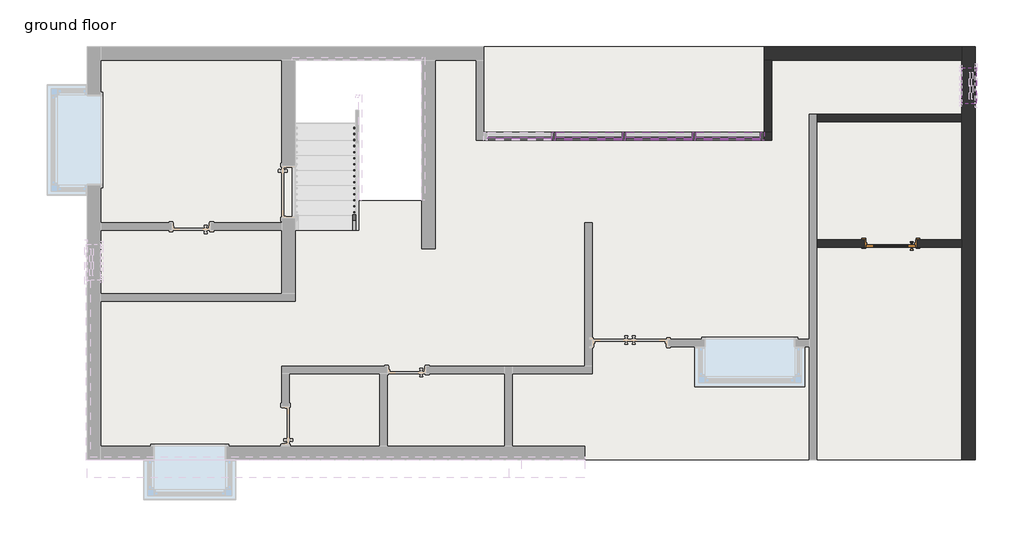
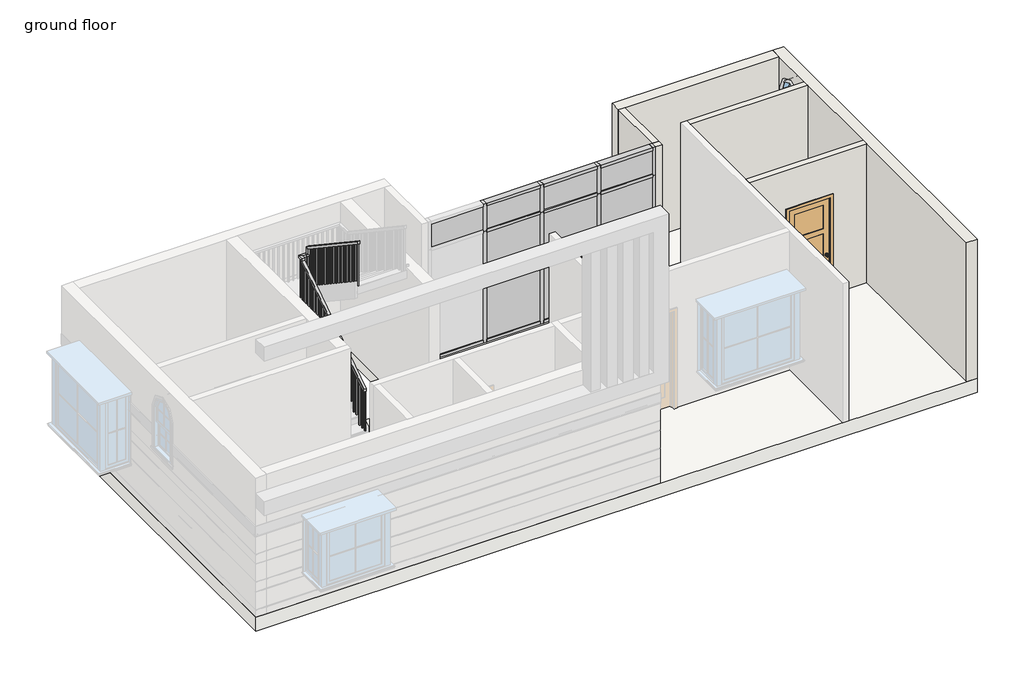
# One storey, part 4 of 5: 18 members, 7 plates, 6 walls, 1 door, 1 railing, 1 slab, 1 window.
"""IFC4 building model written with IfcOpenShell, lengths in millimetres."""

from ifc_helpers import new_model, si_unit, frame, origin, origin_with_axes, place, context, project, spatial, polyline, circle_curve, outline, extrude, faceted_brep, transform, mapped, element, save
from ifc_brep_helpers import plane_surface, revolved_surface, advanced_brep
from components import door_14766595, member_f0fea5a5, member_6e77e263, member_47bfaf8a, member_ee409385, member_5474ae84, member_211d5d53, member_0cc0e230, member_c95c5e6c, system_panel_glazed_91cb7ab6, system_panel_glazed_dcfdf68f, system_panel_glazed_3501c433, system_panel_glazed_b788c8e7, window_777a1d98

model = new_model("IFC4")

# Units and contexts
model_context = context("Model", 3, world=origin())
ifc_project = project(units=[si_unit("LENGTHUNIT", "METRE", prefix="MILLI")], contexts=[model_context])

# Site, building, storey
site = spatial("IfcSite", under=ifc_project)
building = spatial("IfcBuilding", under=site)
storey = spatial("IfcBuildingStorey", under=building, Name="ground floor", Elevation=304.8)

# Door
placement = place(None, origin())
door_shape = door_14766595(model_context)
element("IfcDoor", 1, ObjectType="Door-Interior-Single-3_Panel_Vert-Wood : 33\" x 84\"", at=placement, inside=storey, context=model_context, shape_type="MappedRepresentation", body=[
    mapped(door_shape, transform((359.1327699, -3623.5052427, 304.8), x_axis=(-1.0, 0.0, 0.0), y_axis=(0.0, -1.0, 0.0), z_axis=(0.0, 0.0, 1.0))),
])

# Members
member_shape = member_f0fea5a5(model_context)
element("IfcMember", 2, ObjectType="Rectangular Mullion : 2.5\" x 5\" rectangular", at=placement, inside=storey, context=model_context, shape_type="MappedRepresentation", body=[
    mapped(member_shape, transform((-2955.5672303, -1816.9302427, 304.8), x_axis=(-1.0, 0.0, 0.0), y_axis=(0.0, 1.0, 0.0), z_axis=(0.0, 0.0, -1.0))),
])
element("IfcMember", 3, ObjectType="Rectangular Mullion : 2.5\" x 5\" rectangular", at=placement, inside=storey, context=model_context, shape_type="MappedRepresentation", body=[
    mapped(member_shape, transform((-4136.6672301, -1816.9302427, 304.8), x_axis=(-1.0, 0.0, 0.0), y_axis=(0.0, 1.0, 0.0), z_axis=(0.0, 0.0, -1.0))),
])
element("IfcMember", 4, ObjectType="Rectangular Mullion : 2.5\" x 5\" rectangular", at=placement, inside=storey, context=model_context, shape_type="MappedRepresentation", body=[
    mapped(member_shape, transform((-5317.76723, -1816.9302427, 304.8), x_axis=(-1.0, 0.0, 0.0), y_axis=(0.0, 1.0, 0.0), z_axis=(0.0, 0.0, -1.0))),
])
member_2_shape = member_6e77e263(model_context)
element("IfcMember", 5, ObjectType="Rectangular Mullion : 2.5\" x 5\" rectangular", at=placement, inside=storey, context=model_context, shape_type="MappedRepresentation", body=[
    mapped(member_2_shape, transform((-2955.5672303, -1816.9302427, 2743.2), x_axis=(-1.0, 0.0, 0.0), y_axis=(0.0, 1.0, 0.0), z_axis=(0.0, 0.0, -1.0))),
])
element("IfcMember", 6, ObjectType="Rectangular Mullion : 2.5\" x 5\" rectangular", at=placement, inside=storey, context=model_context, shape_type="MappedRepresentation", body=[
    mapped(member_2_shape, transform((-4136.6672301, -1816.9302427, 2743.2), x_axis=(-1.0, 0.0, 0.0), y_axis=(0.0, 1.0, 0.0), z_axis=(0.0, 0.0, -1.0))),
])
element("IfcMember", 7, ObjectType="Rectangular Mullion : 2.5\" x 5\" rectangular", at=placement, inside=storey, context=model_context, shape_type="MappedRepresentation", body=[
    mapped(member_2_shape, transform((-5317.76723, -1816.9302427, 2743.2), x_axis=(-1.0, 0.0, 0.0), y_axis=(0.0, 1.0, 0.0), z_axis=(0.0, 0.0, -1.0))),
])
member_3_shape = member_47bfaf8a(model_context)
element("IfcMember", 8, ObjectType="Rectangular Mullion : 2.5\" x 5\" rectangular", at=placement, inside=storey, context=model_context, shape_type="MappedRepresentation", body=[
    mapped(member_3_shape, transform((-1774.4672301, -1816.9302427, 3352.8), x_axis=(1.0, 0.0, 0.0), y_axis=(0.0, 1.0, 0.0), z_axis=(0.0, 0.0, 1.0))),
])
member_4_shape = member_ee409385(model_context)
element("IfcMember", 9, ObjectType="Rectangular Mullion : 2.5\" x 5\" rectangular", at=placement, inside=storey, context=model_context, shape_type="MappedRepresentation", body=[
    mapped(member_4_shape, transform((-1774.4672301, -1816.9302427, 2743.2), x_axis=(1.0, 0.0, 0.0), y_axis=(0.0, 1.0, 0.0), z_axis=(0.0, 0.0, 1.0))),
])
member_5_shape = member_5474ae84(model_context)
element("IfcMember", 10, ObjectType="Rectangular Mullion : 2.5\" x 5\" rectangular", at=placement, inside=storey, context=model_context, shape_type="MappedRepresentation", body=[
    mapped(member_5_shape, transform((-2923.8172303, -1816.9302427, 3352.8), x_axis=(0.0, 0.0, 1.0), y_axis=(0.0, 1.0, 0.0), z_axis=(-1.0, 0.0, 0.0))),
])
member_6_shape = member_211d5d53(model_context)
element("IfcMember", 11, ObjectType="Rectangular Mullion : 2.5\" x 5\" rectangular", at=placement, inside=storey, context=model_context, shape_type="MappedRepresentation", body=[
    mapped(member_6_shape, transform((-4104.9172301, -1816.9302427, 3352.8), x_axis=(0.0, 0.0, 1.0), y_axis=(0.0, 1.0, 0.0), z_axis=(-1.0, 0.0, 0.0))),
])
element("IfcMember", 12, ObjectType="Rectangular Mullion : 2.5\" x 5\" rectangular", at=placement, inside=storey, context=model_context, shape_type="MappedRepresentation", body=[
    mapped(member_6_shape, transform((-5286.01723, -1816.9302427, 3352.8), x_axis=(0.0, 0.0, 1.0), y_axis=(0.0, 1.0, 0.0), z_axis=(-1.0, 0.0, 0.0))),
])
element("IfcMember", 13, ObjectType="Rectangular Mullion : 2.5\" x 5\" rectangular", at=placement, inside=storey, context=model_context, shape_type="MappedRepresentation", body=[
    mapped(member_5_shape, transform((-1837.9672301, -1816.9302427, 304.8), x_axis=(0.0, 0.0, -1.0), y_axis=(0.0, 1.0, 0.0), z_axis=(1.0, 0.0, 0.0))),
])
element("IfcMember", 14, ObjectType="Rectangular Mullion : 2.5\" x 5\" rectangular", at=placement, inside=storey, context=model_context, shape_type="MappedRepresentation", body=[
    mapped(member_5_shape, transform((-5349.51723, -1816.9302427, 304.8), x_axis=(0.0, 0.0, -1.0), y_axis=(0.0, 1.0, 0.0), z_axis=(1.0, 0.0, 0.0))),
])
element("IfcMember", 15, ObjectType="Rectangular Mullion : 2.5\" x 5\" rectangular", at=placement, inside=storey, context=model_context, shape_type="MappedRepresentation", body=[
    mapped(member_6_shape, transform((-2987.3172303, -1816.9302427, 304.8), x_axis=(0.0, 0.0, -1.0), y_axis=(0.0, 1.0, 0.0), z_axis=(1.0, 0.0, 0.0))),
])
element("IfcMember", 16, ObjectType="Rectangular Mullion : 2.5\" x 5\" rectangular", at=placement, inside=storey, context=model_context, shape_type="MappedRepresentation", body=[
    mapped(member_6_shape, transform((-4168.4172301, -1816.9302427, 304.8), x_axis=(0.0, 0.0, -1.0), y_axis=(0.0, 1.0, 0.0), z_axis=(1.0, 0.0, 0.0))),
])
member_7_shape = member_0cc0e230(model_context)
element("IfcMember", 17, ObjectType="Rectangular Mullion : 2.5\" x 5\" rectangular", at=placement, inside=storey, context=model_context, shape_type="MappedRepresentation", body=[
    mapped(member_7_shape, transform((-2923.8172303, -1816.9302427, 2743.2), x_axis=(0.0, 0.0, 1.0), y_axis=(0.0, 1.0, 0.0), z_axis=(-1.0, 0.0, 0.0))),
])
member_8_shape = member_c95c5e6c(model_context)
element("IfcMember", 18, ObjectType="Rectangular Mullion : 2.5\" x 5\" rectangular", at=placement, inside=storey, context=model_context, shape_type="MappedRepresentation", body=[
    mapped(member_8_shape, transform((-4104.9172301, -1816.9302427, 2743.2), x_axis=(0.0, 0.0, 1.0), y_axis=(0.0, 1.0, 0.0), z_axis=(-1.0, 0.0, 0.0))),
])
element("IfcMember", 19, ObjectType="Rectangular Mullion : 2.5\" x 5\" rectangular", at=placement, inside=storey, context=model_context, shape_type="MappedRepresentation", body=[
    mapped(member_8_shape, transform((-5286.01723, -1816.9302427, 2743.2), x_axis=(0.0, 0.0, 1.0), y_axis=(0.0, 1.0, 0.0), z_axis=(-1.0, 0.0, 0.0))),
])

# Plates
system_panel_glazed_shape = system_panel_glazed_91cb7ab6(model_context)
element("IfcPlate", 20, ObjectType="System Panel : Glazed", at=placement, inside=storey, context=model_context, shape_type="MappedRepresentation", body=[
    mapped(system_panel_glazed_shape, transform((-2380.8922302, -1816.9302427, 368.3), x_axis=(-1.0, 0.0, 0.0), y_axis=(0.0, -1.0, 0.0), z_axis=(0.0, 0.0, 1.0))),
])
system_panel_glazed_2_shape = system_panel_glazed_dcfdf68f(model_context)
element("IfcPlate", 21, ObjectType="System Panel : Glazed", at=placement, inside=storey, context=model_context, shape_type="MappedRepresentation", body=[
    mapped(system_panel_glazed_2_shape, transform((-3546.1172302, -1816.9302427, 368.3), x_axis=(-1.0, 0.0, 0.0), y_axis=(0.0, -1.0, 0.0), z_axis=(0.0, 0.0, 1.0))),
])
element("IfcPlate", 22, ObjectType="System Panel : Glazed", at=placement, inside=storey, context=model_context, shape_type="MappedRepresentation", body=[
    mapped(system_panel_glazed_2_shape, transform((-4727.21723, -1816.9302427, 368.3), x_axis=(-1.0, 0.0, 0.0), y_axis=(0.0, -1.0, 0.0), z_axis=(0.0, 0.0, 1.0))),
])
system_panel_glazed_3_shape = system_panel_glazed_3501c433(model_context)
element("IfcPlate", 23, ObjectType="System Panel : Glazed", at=placement, inside=storey, context=model_context, shape_type="MappedRepresentation", body=[
    mapped(system_panel_glazed_3_shape, transform((-2380.8922302, -1816.9302427, 2774.95), x_axis=(-1.0, 0.0, 0.0), y_axis=(0.0, -1.0, 0.0), z_axis=(0.0, 0.0, 1.0))),
])
element("IfcPlate", 24, ObjectType="System Panel : Glazed", at=placement, inside=storey, context=model_context, shape_type="MappedRepresentation", body=[
    mapped(system_panel_glazed_3_shape, transform((-5892.44223, -1816.9302427, 2774.95), x_axis=(-1.0, 0.0, 0.0), y_axis=(0.0, -1.0, 0.0), z_axis=(0.0, 0.0, 1.0))),
])
system_panel_glazed_4_shape = system_panel_glazed_b788c8e7(model_context)
element("IfcPlate", 25, ObjectType="System Panel : Glazed", at=placement, inside=storey, context=model_context, shape_type="MappedRepresentation", body=[
    mapped(system_panel_glazed_4_shape, transform((-3546.1172302, -1816.9302427, 2774.95), x_axis=(-1.0, 0.0, 0.0), y_axis=(0.0, -1.0, 0.0), z_axis=(0.0, 0.0, 1.0))),
])
element("IfcPlate", 26, ObjectType="System Panel : Glazed", at=placement, inside=storey, context=model_context, shape_type="MappedRepresentation", body=[
    mapped(system_panel_glazed_4_shape, transform((-4727.21723, -1816.9302427, 2774.95), x_axis=(-1.0, 0.0, 0.0), y_axis=(0.0, -1.0, 0.0), z_axis=(0.0, 0.0, 1.0))),
])

# Railing
element("IfcRailing", 27, ObjectType="Handrail - Rectangular", at=placement, inside=storey, context=model_context, shape_type="SolidModel", body=[
    faceted_brep([(-8708.6672301, -3404.4302427, 1388.5333333), (-8708.6672301, -3404.4302427, 1327.4793317), (-8657.8672301, -3404.4302427, 1327.4793317), (-8657.8672301, -3404.4302427, 1388.5333333), (-8708.6672301, -1194.6302427, 2861.7333333), (-8708.6672301, -1143.8302427, 2834.5459984), (-8657.8672301, -1143.8302427, 2834.5459984), (-8657.8672301, -1194.6302427, 2861.7333333), (-8708.6672301, -1194.6302427, 2912.5333333), (-8708.6672301, -1143.8302427, 2861.7333333), (-8657.8672301, -1143.8302427, 2861.7333333), (-8657.8672301, -1194.6302427, 2912.5333333), (-8708.6672301, -1067.6302427, 2912.5333333), (-8708.6672301, -1067.6302427, 2861.7333333), (-8657.8672301, -1118.4302427, 2861.7333333), (-8657.8672301, -1118.4302427, 2912.5333333), (-8581.6672301, -1067.6302427, 2912.5333333), (-8581.6672301, -1067.6302427, 2861.7333333), (-8581.6672301, -1118.4302427, 2861.7333333), (-8581.6672301, -1118.4302427, 2912.5333333), (-8556.2672301, -1067.6302427, 2912.5333333), (-8556.2672301, -1118.4302427, 2912.5333333), (-8505.4672301, -1118.4302427, 2861.7333333), (-8505.4672301, -1067.6302427, 2861.7333333)], [[[0, 1, 2, 3]], [[1, 0, 4, 5]], [[2, 1, 5, 6]], [[3, 2, 6, 7]], [[0, 3, 7, 4]], [[5, 4, 8, 9]], [[6, 5, 9, 10]], [[7, 6, 10, 11]], [[4, 7, 11, 8]], [[9, 8, 12, 13]], [[10, 9, 13, 14]], [[11, 10, 14, 15]], [[8, 11, 15, 12]], [[13, 12, 16, 17]], [[14, 13, 17, 18]], [[15, 14, 18, 19]], [[12, 15, 19, 16]], [[20, 21, 22, 23]], [[17, 16, 20, 23]], [[18, 17, 23, 22]], [[19, 18, 22, 21]], [[16, 19, 21, 20]]]),
    faceted_brep([(-8556.2672301, -1067.6302427, 2912.5333333), (-8505.4672301, -1067.6302427, 2861.7333333), (-8505.4672301, -1118.4302427, 2861.7333333), (-8556.2672301, -1118.4302427, 2912.5333333), (-8556.2672301, -1067.6302427, 3048.0), (-8556.2672301, -1118.4302427, 3020.8126651), (-8505.4672301, -1118.4302427, 3020.8126651), (-8505.4672301, -1067.6302427, 3048.0)], [[[0, 1, 2, 3]], [[4, 5, 6, 7]], [[1, 0, 4, 7]], [[2, 1, 7, 6]], [[3, 2, 6, 5]], [[0, 3, 5, 4]]]),
    faceted_brep([(-8505.4672301, -1067.6302427, 3048.0), (-8505.4672301, -1118.4302427, 3020.8126651), (-8556.2672301, -1118.4302427, 3020.8126651), (-8556.2672301, -1067.6302427, 3048.0), (-8505.4672301, -2896.4302427, 4267.2), (-8556.2672301, -2896.4302427, 4267.2), (-8556.2672301, -2896.4302427, 4206.1459984), (-8505.4672301, -2896.4302427, 4206.1459984)], [[[0, 1, 2, 3]], [[4, 5, 6, 7]], [[1, 0, 4, 7]], [[2, 1, 7, 6]], [[3, 2, 6, 5]], [[0, 3, 5, 4]]]),
    extrude(outline(polyline([(-2829.7552427, 4161.6959984), (-2810.7052427, 4148.9959984), (-2810.7052427, 3183.4666667), (-2829.7552427, 3183.4666667), (-2829.7552427, 4161.6959984)])), frame((-8540.3922301, 0.0, 0.0), z_axis=(1.0, 0.0, 0.0), x_axis=(0.0, 1.0, 0.0)), (0.0, 0.0, 1.0), 19.05),
    extrude(outline(polyline([(-2728.1552427, 4093.9626651), (-2709.1052427, 4081.2626651), (-2709.1052427, 3183.4666667), (-2728.1552427, 3183.4666667), (-2728.1552427, 4093.9626651)])), frame((-8540.3922301, 0.0, 0.0), z_axis=(1.0, 0.0, 0.0), x_axis=(0.0, 1.0, 0.0)), (0.0, 0.0, 1.0), 19.05),
    extrude(outline(polyline([(-2626.5552427, 4026.2293317), (-2607.5052427, 4013.5293317), (-2607.5052427, 3014.1333333), (-2626.5552427, 3014.1333333), (-2626.5552427, 4026.2293317)])), frame((-8540.3922301, 0.0, 0.0), z_axis=(1.0, 0.0, 0.0), x_axis=(0.0, 1.0, 0.0)), (0.0, 0.0, 1.0), 19.05),
    extrude(outline(polyline([(-2524.9552427, 3958.4959984), (-2505.9052427, 3945.7959984), (-2505.9052427, 3014.1333333), (-2524.9552427, 3014.1333333), (-2524.9552427, 3958.4959984)])), frame((-8540.3922301, 0.0, 0.0), z_axis=(1.0, 0.0, 0.0), x_axis=(0.0, 1.0, 0.0)), (0.0, 0.0, 1.0), 19.05),
    extrude(outline(polyline([(-2423.3552427, 3890.7626651), (-2404.3052427, 3878.0626651), (-2404.3052427, 3014.1333333), (-2423.3552427, 3014.1333333), (-2423.3552427, 3890.7626651)])), frame((-8540.3922301, 0.0, 0.0), z_axis=(1.0, 0.0, 0.0), x_axis=(0.0, 1.0, 0.0)), (0.0, 0.0, 1.0), 19.05),
    extrude(outline(polyline([(-2321.7552427, 3823.0293317), (-2302.7052427, 3810.3293317), (-2302.7052427, 2844.8), (-2321.7552427, 2844.8), (-2321.7552427, 3823.0293317)])), frame((-8540.3922301, 0.0, 0.0), z_axis=(1.0, 0.0, 0.0), x_axis=(0.0, 1.0, 0.0)), (0.0, 0.0, 1.0), 19.05),
    extrude(outline(polyline([(-2220.1552427, 3755.2959984), (-2201.1052427, 3742.5959984), (-2201.1052427, 2844.8), (-2220.1552427, 2844.8), (-2220.1552427, 3755.2959984)])), frame((-8540.3922301, 0.0, 0.0), z_axis=(1.0, 0.0, 0.0), x_axis=(0.0, 1.0, 0.0)), (0.0, 0.0, 1.0), 19.05),
    extrude(outline(polyline([(-2118.5552427, 3687.5626651), (-2099.5052427, 3674.8626651), (-2099.5052427, 2675.4666667), (-2118.5552427, 2675.4666667), (-2118.5552427, 3687.5626651)])), frame((-8540.3922301, 0.0, 0.0), z_axis=(1.0, 0.0, 0.0), x_axis=(0.0, 1.0, 0.0)), (0.0, 0.0, 1.0), 19.05),
    extrude(outline(polyline([(-2016.9552427, 3619.8293317), (-1997.9052427, 3607.1293317), (-1997.9052427, 2675.4666667), (-2016.9552427, 2675.4666667), (-2016.9552427, 3619.8293317)])), frame((-8540.3922301, 0.0, 0.0), z_axis=(1.0, 0.0, 0.0), x_axis=(0.0, 1.0, 0.0)), (0.0, 0.0, 1.0), 19.05),
    extrude(outline(polyline([(-1915.3552427, 3552.0959984), (-1896.3052427, 3539.3959984), (-1896.3052427, 2675.4666667), (-1915.3552427, 2675.4666667), (-1915.3552427, 3552.0959984)])), frame((-8540.3922301, 0.0, 0.0), z_axis=(1.0, 0.0, 0.0), x_axis=(0.0, 1.0, 0.0)), (0.0, 0.0, 1.0), 19.05),
    extrude(outline(polyline([(-1813.7552427, 3484.3626651), (-1794.7052427, 3471.6626651), (-1794.7052427, 2506.1333333), (-1813.7552427, 2506.1333333), (-1813.7552427, 3484.3626651)])), frame((-8540.3922301, 0.0, 0.0), z_axis=(1.0, 0.0, 0.0), x_axis=(0.0, 1.0, 0.0)), (0.0, 0.0, 1.0), 19.05),
    extrude(outline(polyline([(-1712.1552427, 3416.6293317), (-1693.1052427, 3403.9293317), (-1693.1052427, 2506.1333333), (-1712.1552427, 2506.1333333), (-1712.1552427, 3416.6293317)])), frame((-8540.3922301, 0.0, 0.0), z_axis=(1.0, 0.0, 0.0), x_axis=(0.0, 1.0, 0.0)), (0.0, 0.0, 1.0), 19.05),
    extrude(outline(polyline([(-1610.5552427, 3348.8959984), (-1591.5052427, 3336.1959984), (-1591.5052427, 2336.8), (-1610.5552427, 2336.8), (-1610.5552427, 3348.8959984)])), frame((-8540.3922301, 0.0, 0.0), z_axis=(1.0, 0.0, 0.0), x_axis=(0.0, 1.0, 0.0)), (0.0, 0.0, 1.0), 19.05),
    extrude(outline(polyline([(-1508.9552427, 3281.1626651), (-1489.9052427, 3268.4626651), (-1489.9052427, 2336.8), (-1508.9552427, 2336.8), (-1508.9552427, 3281.1626651)])), frame((-8540.3922301, 0.0, 0.0), z_axis=(1.0, 0.0, 0.0), x_axis=(0.0, 1.0, 0.0)), (0.0, 0.0, 1.0), 19.05),
    extrude(outline(polyline([(-1407.3552427, 3213.4293317), (-1388.3052427, 3200.7293317), (-1388.3052427, 2336.8), (-1407.3552427, 2336.8), (-1407.3552427, 3213.4293317)])), frame((-8540.3922301, 0.0, 0.0), z_axis=(1.0, 0.0, 0.0), x_axis=(0.0, 1.0, 0.0)), (0.0, 0.0, 1.0), 19.05),
    extrude(outline(polyline([(-1305.7552427, 3145.6959984), (-1286.7052427, 3132.9959984), (-1286.7052427, 2167.4666667), (-1305.7552427, 2167.4666667), (-1305.7552427, 3145.6959984)])), frame((-8540.3922301, 0.0, 0.0), z_axis=(1.0, 0.0, 0.0), x_axis=(0.0, 1.0, 0.0)), (0.0, 0.0, 1.0), 19.05),
    extrude(outline(polyline([(-1204.1552427, 3077.9626651), (-1185.1052427, 3065.2626651), (-1185.1052427, 2167.4666667), (-1204.1552427, 2167.4666667), (-1204.1552427, 3077.9626651)])), frame((-8540.3922301, 0.0, 0.0), z_axis=(1.0, 0.0, 0.0), x_axis=(0.0, 1.0, 0.0)), (0.0, 0.0, 1.0), 19.05),
    extrude(outline(polyline([(-8591.1922301, -1102.5552427), (-8591.1922301, -1083.5052427), (-8572.1422301, -1083.5052427), (-8572.1422301, -1102.5552427), (-8591.1922301, -1102.5552427)])), frame((0.0, 0.0, 1998.1333333), z_axis=(0.0, 0.0, 1.0), x_axis=(1.0, 0.0, 0.0)), (0.0, 0.0, 1.0), 863.6),
    extrude(outline(polyline([(-8673.7422301, -1178.7552427), (-8692.7922301, -1178.7552427), (-8692.7922301, -1159.7052427), (-8673.7422301, -1159.7052427), (-8673.7422301, -1178.7552427)])), frame((0.0, 0.0, 1828.8), z_axis=(0.0, 0.0, 1.0), x_axis=(1.0, 0.0, 0.0)), (0.0, 0.0, 1.0), 1032.9333333),
    extrude(outline(polyline([(-1280.3552427, 2743.5293317), (-1261.3052427, 2756.2293317), (-1261.3052427, 1828.8), (-1280.3552427, 1828.8), (-1280.3552427, 2743.5293317)])), frame((-8692.7922301, 0.0, 0.0), z_axis=(1.0, 0.0, 0.0), x_axis=(0.0, 1.0, 0.0)), (0.0, 0.0, 1.0), 19.05),
    extrude(outline(polyline([(-1381.9552427, 2675.7959984), (-1362.9052427, 2688.4959984), (-1362.9052427, 1828.8), (-1381.9552427, 1828.8), (-1381.9552427, 2675.7959984)])), frame((-8692.7922301, 0.0, 0.0), z_axis=(1.0, 0.0, 0.0), x_axis=(0.0, 1.0, 0.0)), (0.0, 0.0, 1.0), 19.05),
    extrude(outline(polyline([(-1483.5552427, 2608.0626651), (-1464.5052427, 2620.7626651), (-1464.5052427, 1659.4666667), (-1483.5552427, 1659.4666667), (-1483.5552427, 2608.0626651)])), frame((-8692.7922301, 0.0, 0.0), z_axis=(1.0, 0.0, 0.0), x_axis=(0.0, 1.0, 0.0)), (0.0, 0.0, 1.0), 19.05),
    extrude(outline(polyline([(-1585.1552427, 2540.3293317), (-1566.1052427, 2553.0293317), (-1566.1052427, 1659.4666667), (-1585.1552427, 1659.4666667), (-1585.1552427, 2540.3293317)])), frame((-8692.7922301, 0.0, 0.0), z_axis=(1.0, 0.0, 0.0), x_axis=(0.0, 1.0, 0.0)), (0.0, 0.0, 1.0), 19.05),
    extrude(outline(polyline([(-1686.7552427, 2472.5959984), (-1667.7052427, 2485.2959984), (-1667.7052427, 1490.1333333), (-1686.7552427, 1490.1333333), (-1686.7552427, 2472.5959984)])), frame((-8692.7922301, 0.0, 0.0), z_axis=(1.0, 0.0, 0.0), x_axis=(0.0, 1.0, 0.0)), (0.0, 0.0, 1.0), 19.05),
    extrude(outline(polyline([(-1788.3552427, 2404.8626651), (-1769.3052427, 2417.5626651), (-1769.3052427, 1490.1333333), (-1788.3552427, 1490.1333333), (-1788.3552427, 2404.8626651)])), frame((-8692.7922301, 0.0, 0.0), z_axis=(1.0, 0.0, 0.0), x_axis=(0.0, 1.0, 0.0)), (0.0, 0.0, 1.0), 19.05),
    extrude(outline(polyline([(-1889.9552427, 2337.1293317), (-1870.9052427, 2349.8293317), (-1870.9052427, 1490.1333333), (-1889.9552427, 1490.1333333), (-1889.9552427, 2337.1293317)])), frame((-8692.7922301, 0.0, 0.0), z_axis=(1.0, 0.0, 0.0), x_axis=(0.0, 1.0, 0.0)), (0.0, 0.0, 1.0), 19.05),
    extrude(outline(polyline([(-1991.5552427, 2269.3959984), (-1972.5052427, 2282.0959984), (-1972.5052427, 1320.8), (-1991.5552427, 1320.8), (-1991.5552427, 2269.3959984)])), frame((-8692.7922301, 0.0, 0.0), z_axis=(1.0, 0.0, 0.0), x_axis=(0.0, 1.0, 0.0)), (0.0, 0.0, 1.0), 19.05),
    extrude(outline(polyline([(-2093.1552427, 2201.6626651), (-2074.1052427, 2214.3626651), (-2074.1052427, 1320.8), (-2093.1552427, 1320.8), (-2093.1552427, 2201.6626651)])), frame((-8692.7922301, 0.0, 0.0), z_axis=(1.0, 0.0, 0.0), x_axis=(0.0, 1.0, 0.0)), (0.0, 0.0, 1.0), 19.05),
    extrude(outline(polyline([(-2194.7552427, 2133.9293317), (-2175.7052427, 2146.6293317), (-2175.7052427, 1151.4666667), (-2194.7552427, 1151.4666667), (-2194.7552427, 2133.9293317)])), frame((-8692.7922301, 0.0, 0.0), z_axis=(1.0, 0.0, 0.0), x_axis=(0.0, 1.0, 0.0)), (0.0, 0.0, 1.0), 19.05),
    extrude(outline(polyline([(-2296.3552427, 2066.1959984), (-2277.3052427, 2078.8959984), (-2277.3052427, 1151.4666667), (-2296.3552427, 1151.4666667), (-2296.3552427, 2066.1959984)])), frame((-8692.7922301, 0.0, 0.0), z_axis=(1.0, 0.0, 0.0), x_axis=(0.0, 1.0, 0.0)), (0.0, 0.0, 1.0), 19.05),
    extrude(outline(polyline([(-2397.9552427, 1998.4626651), (-2378.9052427, 2011.1626651), (-2378.9052427, 1151.4666667), (-2397.9552427, 1151.4666667), (-2397.9552427, 1998.4626651)])), frame((-8692.7922301, 0.0, 0.0), z_axis=(1.0, 0.0, 0.0), x_axis=(0.0, 1.0, 0.0)), (0.0, 0.0, 1.0), 19.05),
    extrude(outline(polyline([(-2499.5552427, 1930.7293317), (-2480.5052427, 1943.4293317), (-2480.5052427, 982.1333333), (-2499.5552427, 982.1333333), (-2499.5552427, 1930.7293317)])), frame((-8692.7922301, 0.0, 0.0), z_axis=(1.0, 0.0, 0.0), x_axis=(0.0, 1.0, 0.0)), (0.0, 0.0, 1.0), 19.05),
    extrude(outline(polyline([(-2601.1552427, 1862.9959984), (-2582.1052427, 1875.6959984), (-2582.1052427, 982.1333333), (-2601.1552427, 982.1333333), (-2601.1552427, 1862.9959984)])), frame((-8692.7922301, 0.0, 0.0), z_axis=(1.0, 0.0, 0.0), x_axis=(0.0, 1.0, 0.0)), (0.0, 0.0, 1.0), 19.05),
    extrude(outline(polyline([(-2702.7552427, 1795.2626651), (-2683.7052427, 1807.9626651), (-2683.7052427, 812.8), (-2702.7552427, 812.8), (-2702.7552427, 1795.2626651)])), frame((-8692.7922301, 0.0, 0.0), z_axis=(1.0, 0.0, 0.0), x_axis=(0.0, 1.0, 0.0)), (0.0, 0.0, 1.0), 19.05),
    extrude(outline(polyline([(-2804.3552427, 1727.5293317), (-2785.3052427, 1740.2293317), (-2785.3052427, 812.8), (-2804.3552427, 812.8), (-2804.3552427, 1727.5293317)])), frame((-8692.7922301, 0.0, 0.0), z_axis=(1.0, 0.0, 0.0), x_axis=(0.0, 1.0, 0.0)), (0.0, 0.0, 1.0), 19.05),
    extrude(outline(polyline([(-2905.9552427, 1659.7959984), (-2886.9052427, 1672.4959984), (-2886.9052427, 812.8), (-2905.9552427, 812.8), (-2905.9552427, 1659.7959984)])), frame((-8692.7922301, 0.0, 0.0), z_axis=(1.0, 0.0, 0.0), x_axis=(0.0, 1.0, 0.0)), (0.0, 0.0, 1.0), 19.05),
    extrude(outline(polyline([(-3007.5552427, 1592.0626651), (-2988.5052427, 1604.7626651), (-2988.5052427, 643.4666667), (-3007.5552427, 643.4666667), (-3007.5552427, 1592.0626651)])), frame((-8692.7922301, 0.0, 0.0), z_axis=(1.0, 0.0, 0.0), x_axis=(0.0, 1.0, 0.0)), (0.0, 0.0, 1.0), 19.05),
    extrude(outline(polyline([(-3109.1552427, 1524.3293317), (-3090.1052427, 1537.0293317), (-3090.1052427, 643.4666667), (-3109.1552427, 643.4666667), (-3109.1552427, 1524.3293317)])), frame((-8692.7922301, 0.0, 0.0), z_axis=(1.0, 0.0, 0.0), x_axis=(0.0, 1.0, 0.0)), (0.0, 0.0, 1.0), 19.05),
    extrude(outline(polyline([(-3210.7552427, 1456.5959984), (-3191.7052427, 1469.2959984), (-3191.7052427, 474.1333333), (-3210.7552427, 474.1333333), (-3210.7552427, 1456.5959984)])), frame((-8692.7922301, 0.0, 0.0), z_axis=(1.0, 0.0, 0.0), x_axis=(0.0, 1.0, 0.0)), (0.0, 0.0, 1.0), 19.05),
    extrude(outline(polyline([(-3312.3552427, 1388.8626651), (-3293.3052427, 1401.5626651), (-3293.3052427, 474.1333333), (-3312.3552427, 474.1333333), (-3312.3552427, 1388.8626651)])), frame((-8692.7922301, 0.0, 0.0), z_axis=(1.0, 0.0, 0.0), x_axis=(0.0, 1.0, 0.0)), (0.0, 0.0, 1.0), 19.05),
    extrude(outline(polyline([(-8540.3922301, -1102.5552427), (-8540.3922301, -1083.5052427), (-8521.3422301, -1083.5052427), (-8521.3422301, -1102.5552427), (-8540.3922301, -1102.5552427)])), frame((0.0, 0.0, 1998.1333333), z_axis=(0.0, 0.0, 1.0), x_axis=(1.0, 0.0, 0.0)), (0.0, 0.0, 1.0), 863.6),
    extrude(outline(polyline([(-8673.7422301, -1102.5552427), (-8692.7922301, -1102.5552427), (-8692.7922301, -1083.5052427), (-8673.7422301, -1083.5052427), (-8673.7422301, -1102.5552427)])), frame((0.0, 0.0, 1998.1333333), z_axis=(0.0, 0.0, 1.0), x_axis=(1.0, 0.0, 0.0)), (0.0, 0.0, 1.0), 863.6),
    extrude(outline(polyline([(-2896.4302427, 4206.1459984), (-2877.3802427, 4193.4459984), (-2877.3802427, 3183.4666667), (-2896.4302427, 3183.4666667), (-2896.4302427, 4206.1459984)])), frame((-8540.3922301, 0.0, 0.0), z_axis=(1.0, 0.0, 0.0), x_axis=(0.0, 1.0, 0.0)), (0.0, 0.0, 1.0), 19.05),
    extrude(outline(polyline([(-3404.4302427, 1327.4793317), (-3385.3802427, 1340.1793317), (-3385.3802427, 474.1333333), (-3404.4302427, 474.1333333), (-3404.4302427, 1327.4793317)])), frame((-8692.7922301, 0.0, 0.0), z_axis=(1.0, 0.0, 0.0), x_axis=(0.0, 1.0, 0.0)), (0.0, 0.0, 1.0), 19.05),
])

# Slab
element("IfcSlab", 28, ObjectType="Generic - 12\"", at=placement, inside=storey, context=model_context, shape_type="SweptSolid", body=[
    extrude(outline(polyline([(1781.5327699, -305.6302427), (1781.5327699, -7265.2302427), (-13179.0672301, -7265.2302427), (-13179.0672301, -305.6302427), (1781.5327699, -305.6302427)]), holes=[polyline([(-9724.6672301, -3379.0302427), (-8607.0672301, -3404.4302427), (-8607.0672301, -2896.4302427), (-7489.4672301, -2896.4302427), (-7489.4672301, -483.4302427), (-9724.6672301, -483.4302427), (-9724.6672301, -3379.0302427)])]), origin_with_axes(), (0.0, 0.0, 1.0), 304.8),
])

# Walls
element("IfcWall", 29, ObjectType="INNER WALL 5\"", at=placement, inside=storey, context=model_context, shape_type="SweptSolid", body=[
    extrude(outline(polyline([(1552.9327699, -1575.6302427), (-885.4672301, -1575.6302427), (-885.4672301, -1448.6302427), (1552.9327699, -1448.6302427), (1552.9327699, -1575.6302427)])), frame((0.0, 0.0, 304.8), z_axis=(0.0, 0.0, 1.0), x_axis=(1.0, 0.0, 0.0)), (0.0, 0.0, 1.0), 3048.0),
])
element("IfcWall", 30, ObjectType="INNER WALL 5\"", at=placement, inside=storey, context=model_context, shape_type="SweptSolid", body=[
    extrude(outline(polyline([(3352.8, 1552.9327699), (3352.8, -885.4672301), (304.8, -885.4672301), (304.8, -85.3672301), (2463.8, -85.3672301), (2463.8, 803.6327699), (304.8, 803.6327699), (304.8, 1552.9327699), (3352.8, 1552.9327699)])), frame((0.0, -3683.8302427, 0.0), z_axis=(0.0, 1.0, 0.0), x_axis=(0.0, 0.0, 1.0)), (0.0, 0.0, 1.0), 127.0),
])
element("IfcWall", 31, ObjectType="INNER WALL 5\"", at=placement, inside=storey, context=model_context, shape_type="SweptSolid", body=[
    extrude(outline(polyline([(-1647.4672301, -1753.4302427), (-1647.4672301, -1880.4302427), (-1774.4672301, -1880.4302427), (-1774.4672301, -1753.4302427), (-1647.4672301, -1753.4302427)])), frame((0.0, 0.0, 304.8), z_axis=(0.0, 0.0, 1.0), x_axis=(1.0, 0.0, 0.0)), (0.0, 0.0, 1.0), 3048.0),
])
element("IfcWall", 32, ObjectType="INNER WALL 5\"", at=placement, inside=storey, context=model_context, shape_type="SweptSolid", body=[
    extrude(outline(polyline([(-1647.4672301, -534.2302427), (-1647.4672301, -1753.4302427), (-1774.4672301, -1753.4302427), (-1774.4672301, -534.2302427), (-1647.4672301, -534.2302427)])), frame((0.0, 0.0, 304.8), z_axis=(0.0, 0.0, 1.0), x_axis=(1.0, 0.0, 0.0)), (0.0, 0.0, 1.0), 3048.0),
])
element("IfcWall", 33, ObjectType="OUTER WALL 9\"", at=placement, inside=storey, context=model_context, shape_type="AdvancedBrep", body=[
    advanced_brep(
    [(1781.5327699, -7265.2302427, 304.8), (1781.5327699, -305.6302427, 304.8), (1781.5327699, -305.6302427, 3352.8), (1781.5327699, -7265.2302427, 3352.8), (1781.5327699, -1270.8302427, 2743.2), (1781.5327699, -661.2302427, 2743.2), (1781.5327699, -661.2302427, 1828.8), (1781.5327699, -1270.8302427, 1828.8), (1552.9327699, -7265.2302427, 304.8), (1552.9327699, -7265.2302427, 3352.8), (1552.9327699, -3683.8302427, 3352.8), (1552.9327699, -3556.8302427, 3352.8), (1552.9327699, -1575.6302427, 3352.8), (1552.9327699, -1448.6302427, 3352.8), (1552.9327699, -534.2302427, 3352.8), (1552.9327699, -305.6302427, 3352.8), (1552.9327699, -305.6302427, 304.8), (1552.9327699, -534.2302427, 304.8), (1552.9327699, -1448.6302427, 304.8), (1552.9327699, -1575.6302427, 304.8), (1552.9327699, -3556.8302427, 304.8), (1552.9327699, -3683.8302427, 304.8), (1552.9327699, -1270.8302427, 2743.2), (1552.9327699, -1270.8302427, 1828.8), (1552.9327699, -661.2302427, 1828.8), (1552.9327699, -661.2302427, 2743.2)],
    [
        (0, 1),
        (1, 2),
        (2, 3),
        (3, 0),
        (4, 5, circle_curve(frame((1781.5327699, -966.0302427, 2743.2), z_axis=(-1.0, 0.0, 0.0), x_axis=(0.0, -1.0, 0.0)), 304.8)),
        (5, 6),
        (6, 7),
        (7, 4),
        (8, 9),
        (9, 10),
        (10, 11),
        (11, 12),
        (12, 13),
        (13, 14),
        (14, 15),
        (15, 16),
        (16, 17),
        (17, 18),
        (18, 19),
        (19, 20),
        (20, 21),
        (21, 8),
        (22, 23),
        (23, 24),
        (24, 25),
        (25, 22, circle_curve(frame((1552.9327699, -966.0302427, 2743.2), z_axis=(1.0, 0.0, 0.0), x_axis=(0.0, -1.0, 0.0)), 304.8)),
        (0, 8),
        (16, 1),
        (2, 15),
        (9, 3),
        (4, 22),
        (25, 5),
        (24, 6),
        (23, 7),
    ],
    [
        plane_surface(frame((1781.5327699, -7257.9419141, 304.8), z_axis=(1.0, 0.0, 0.0), x_axis=(0.0, 1.0, 0.0))),
        plane_surface(frame((1552.9327699, -7257.9419141, 304.8), z_axis=(-1.0, 0.0, 0.0), x_axis=(0.0, -1.0, 0.0))),
        plane_surface(frame((1781.5327699, -7265.2302427, 304.8), z_axis=(0.0, 0.0, -1.0), x_axis=(-1.0, 0.0, 0.0))),
        plane_surface(frame((1781.5327699, -419.9302427, 3352.8), z_axis=(0.0, 0.0, 1.0), x_axis=(-1.0, 0.0, 0.0))),
        plane_surface(frame((1781.5327699, -7265.2302427, 3352.8), z_axis=(0.0, -1.0, 0.0), x_axis=(-1.0, 0.0, 0.0))),
        plane_surface(frame((1781.5327699, -305.6302427, 304.8), z_axis=(0.0, 1.0, 0.0), x_axis=(-1.0, 0.0, 0.0))),
        revolved_surface(polyline([(1552.9327699, -1270.8302427, 2743.2), (1781.5327699, -1270.8302427, 2743.2)]), (1552.9327699, -966.0302427, 2743.2), (-1.0, 0.0, 0.0)),
        plane_surface(frame((1781.5327699, -661.2302427, 2743.2), z_axis=(0.0, -1.0, 0.0), x_axis=(-1.0, 0.0, 0.0))),
        plane_surface(frame((1781.5327699, -661.2302427, 1828.8), z_axis=(0.0, 0.0, 1.0), x_axis=(-1.0, 0.0, 0.0))),
        plane_surface(frame((1781.5327699, -1270.8302427, 1828.8), z_axis=(0.0, 1.0, 0.0), x_axis=(-1.0, 0.0, 0.0))),
    ],
    [
        (0, [[1, 2, 3, 4], [5, 6, 7, 8]]),
        (1, [[9, 10, 11, 12, 13, 14, 15, 16, 17, 18, 19, 20, 21, 22], [23, 24, 25, 26]]),
        (2, [[-1, 27, -22, -21, -20, -19, -18, -17, 28]]),
        (3, [[-3, 29, -15, -14, -13, -12, -11, -10, 30]]),
        (4, [[-4, -30, -9, -27]]),
        (5, [[-2, -28, -16, -29]]),
        (6, [[-5, 31, -26, 32]]),
        (7, [[-6, -32, -25, 33]]),
        (8, [[-7, -33, -24, 34]]),
        (9, [[-8, -34, -23, -31]]),
    ],
),
])
element("IfcWall", 34, ObjectType="OUTER WALL 9\"", at=placement, inside=storey, context=model_context, shape_type="Brep", body=[
    faceted_brep([(1552.9327699, -305.6302427, 304.8), (-1774.4672301, -305.6302427, 304.8), (-1774.4672301, -305.6302427, 3352.8), (1552.9327699, -305.6302427, 3352.8), (1552.9327699, -534.2302427, 304.8), (1552.9327699, -534.2302427, 3352.8), (-1647.4672301, -534.2302427, 3352.8), (-1774.4672301, -534.2302427, 3352.8), (-1774.4672301, -534.2302427, 304.8), (-1647.4672301, -534.2302427, 304.8)], [[[0, 1, 2, 3]], [[4, 5, 6, 7, 8, 9]], [[1, 0, 4, 9, 8]], [[3, 2, 7, 6, 5]], [[0, 3, 5, 4]], [[2, 1, 8, 7]]]),
])

# Window
window_shape = window_777a1d98(model_context)
element("IfcWindow", 35, ObjectType="Window-Double-Hung-Arch-Head : 24\" x 48\"", at=placement, inside=storey, context=model_context, shape_type="MappedRepresentation", body=[
    mapped(window_shape, transform((1667.2327699, -966.0302427, 914.4), x_axis=(0.0, -1.0, 0.0), y_axis=(1.0, 0.0, 0.0), z_axis=(0.0, 0.0, 1.0))),
])

save(model, "model.ifc")

# Revit data of these elements
# Type "Door-Interior-Single-3_Panel_Vert-Wood : 33\" x 84\""
#   Type Mark = "11"
#   Assembly Code = "C1020300"
#   Analytic Construction = "Wooden"
#   Top Rail = 0' - 4 11/16"
#   Thickness = 0' - 1 3/8"
#   Thermal Resistance (R) = 2.5876 (h·ft²·°F)/BTU
#   Swing Angle [instance default] = 90.00°
#   Stiles = 0' - 4 3/4"
#   Rough Width = 2' - 11"
#   Rough Height = 7' - 1"
#   Intermediate Rail = 0' - 4 1/2"
#   Height = 7' - 0"
#   Width = 2' - 9"
#   Heat Transfer Coefficient (U) = 0.3865 BTU/(h·ft²·°F)
#   Bottom Rail = 0' - 9 1/8"
#   Trim Material = Cherry
#   Panel Material = Cherry
#   Frame Material = Cherry
#   Door Handle Material = Aluminum
#   Visual Light Transmittance = 0
#   Solar Heat Gain Coefficient = 0
#   Wall Closure = (empty or 0)
#   Function = (empty or 0)
# Type "Rectangular Mullion : 2.5\" x 5\" rectangular"
#   built-in parameter 1007304 = 0.416667 (stored number, unit not read)
#   built-in parameter 1007301 = 0.104167 (stored number, unit not read)
#   built-in parameter 1007300 = 0.104167 (stored number, unit not read)
# Type "System Panel : Glazed"
#   Construction Type Id = "GSP4R"
#   Analytic Construction = "1/8 in Pilkington single glazing"
#   Visual Light Transmittance = 0.9
#   Solar Heat Gain Coefficient = 0.86
#   Heat Transfer Coefficient (U) = 1.18115 BTU/(h·ft²·°F)
#   Define Thermal Properties by = 1
# Type "Handrail - Rectangular"
#   Assembly Code = "C2010400"
#   built-in parameter 1008612 = 0.0416667 (stored number, unit not read)
#   built-in parameter 1008611 = 0.0416667 (stored number, unit not read)
#   built-in parameter 1008609 = 0.333333 (stored number, unit not read)
#   built-in parameter 1008604 = 0.166667 (stored number, unit not read)
#   built-in parameter 1008603 = 0.166667 (stored number, unit not read)
#   Railing Height = 3' - 0"
#   built-in parameter 1008630 = 2
#   built-in parameter 1008610 = 2
#   built-in parameter 1008618 = Baluster - Square : 3/4"
# Type "Generic - 12\""
#   Assembly Code = "B1010"
#   Function = 0
#   Layers, outside or top first: 1' - 0" "MARBLE FLOORING" (function 1)
# Type "INNER WALL 5\""
#   Assembly Code = "B2010"
#   Layers, outside or top first: 0' - 5" "WARM BEIGE COLOUR" (function 1)
# Type "OUTER WALL 9\""
#   Assembly Code = "B2010"
#   Layers, outside or top first: 0' - 9" "WARM BEIGE COLOUR" (function 1)
# Type "Window-Double-Hung-Arch-Head : 24\" x 48\""
#   Type Mark = "19"
#   Fire Rating = "0.5h"
#   Construction Type Id = "DG-DR"
#   Assembly Code = "B2020100"
#   Analytic Construction = "Double glazing - domestic"
#   Wall Thickness [instance default] = 0' - 6"
#   Window Inset [instance default] = 0' - 0"
#   Visual Light Transmittance = 0.81
#   Thermal Resistance (R) = 1.8146 (h·ft²·°F)/BTU
#   Solar Heat Gain Coefficient = 0.76
#   Muntin Width = 1' - 6"
#   Muntin Height = 1' - 8 1/8"
#   Interior Wall Closure [instance default] = 0' - 1 1/2"
#   Rough Width = 2' - 0 1/2"
#   Rough Height = 4' - 0 1/2"
#   Half Width = 1' - 0"
#   Frame Extension [instance default] = 0' - 1 1/4"
#   Exterior Wall Closure [instance default] = 0' - 0 1/2"
#   Extension Jamb [instance default] = 0' - 1 1/2"
#   Heat Transfer Coefficient (U) = 0.5511 BTU/(h·ft²·°F)
#   Height = 4' - 0"
#   Width = 2' - 0"
#   Top Muntin Visibility = yes
#   Indicator Visibility [instance default] = yes
#   Extension Jamb Visibility [instance default] = yes
#   Interior Trim Visibility [instance default] = yes
#   Exterior Trim Visibility [instance default] = yes
#   Define Thermal Properties by = 1
#   Bottom Muntin Visibility = yes
#   Muntin Pattern = Muntin Pattern_2x2 : Muntin Pattern_2x2
#   Interior Trim Material = Wood - Stained
#   Interior Trim = Trim-Window-Interior-Arch-Hung : Picture Frame
#   Exterior Trim Material = Clad - White
#   Exterior Trim = Trim-Window-Exterior-Arch-Hung : with Sill
#   Glass Panel Material = Glass
#   Exterior Frame Material = Clad - White
#   Interior Frame Material = Wood - Stained
#   Wall Closure = (empty or 0)
# Element 1 (IfcDoor, "Door-Interior-Single-3_Panel_Vert-Wood : 33\" x 84\"")
#   Swing Angle = 90.00°
#   Phase Created = New Construction
#   Materials on its faces: "Cherry", "Aluminum"
# Elements 2, 3, 4, 5, 6, 7, 8, 9, 10, 11, 12, 13, 14, 15, 16, 17, 18, 19 (IfcMember, "Rectangular Mullion : 2.5\" x 5\" rectangular")
#   Phase Created = New Construction
#   Materials on its faces: "Aluminum"
# Elements 20, 21, 22, 23, 24, 25, 26 (IfcPlate, "System Panel : Glazed")
#   Phase Created = New Construction
#   Materials on its faces: "Glass"
# Element 27 (IfcRailing, "Handrail - Rectangular")
#   Phase Created = New Construction
# Element 28 (IfcSlab, "Generic - 12\"")
#   Height Offset From Level = 0' - 0"
#   Phase Created = New Construction
#   Materials on its faces: "MARBLE FLOORING"
# Elements 29, 30, 31, 32 (IfcWall, "INNER WALL 5\"")
#   Top Offset = 0' - 0"
#   Base Offset = 0' - 0"
#   wall height = 10' - 0"
#   Phase Created = New Construction
#   Base Constraint = ground floor
#   Top Constraint = first floor
#   Materials on its faces: "WARM BEIGE COLOUR"
# Elements 33, 34 (IfcWall, "OUTER WALL 9\"")
#   Top Offset = 0' - 0"
#   Base Offset = 0' - 0"
#   wall height = 10' - 0"
#   Phase Created = New Construction
#   Base Constraint = ground floor
#   Top Constraint = first floor
#   Materials on its faces: "WARM BEIGE COLOUR"
# Element 35 (IfcWindow, "Window-Double-Hung-Arch-Head : 24\" x 48\"")
#   Mark = "4"
#   Window Inset = 0' - 0"
#   Interior Wall Closure = 0' - 1 1/2"
#   Frame Extension = 0' - 1 1/4"
#   Exterior Wall Closure = 0' - 0 1/2"
#   Interior Trim Visibility = yes
#   Indicator Visibility = yes
#   Exterior Trim Visibility = yes
#   Phase Created = New Construction
#   Materials on its faces: "Wood - Stained", "Glass", "Clad - White"
# Materials
#   "Cherry": class "Wood", colour RGB 226 177 128, transparency 0, Description = "Prunus Serotina", Cost = 0
#   "Aluminum": class "Metal", colour RGB 247 247 247, transparency 0, Description = "Aluminum 6061", Cost = 0
#   "MARBLE FLOORING": class "Generic", colour RGB 120 120 120, transparency 0, Cost = 0
#   "WARM BEIGE COLOUR": class "Generic", colour RGB 120 120 120, transparency 0, Cost = 0
#   "Wood - Stained": class "Wood", colour RGB 224 178 126, transparency 0, Cost = 0
#   "Clad - White": class "Wood", colour RGB 242 242 238, transparency 0, Cost = 0
#   "Glass": class "Glass", colour RGB 0 128 192, transparency 0.75, Description = "Soda Lime Glass", Cost = 0
